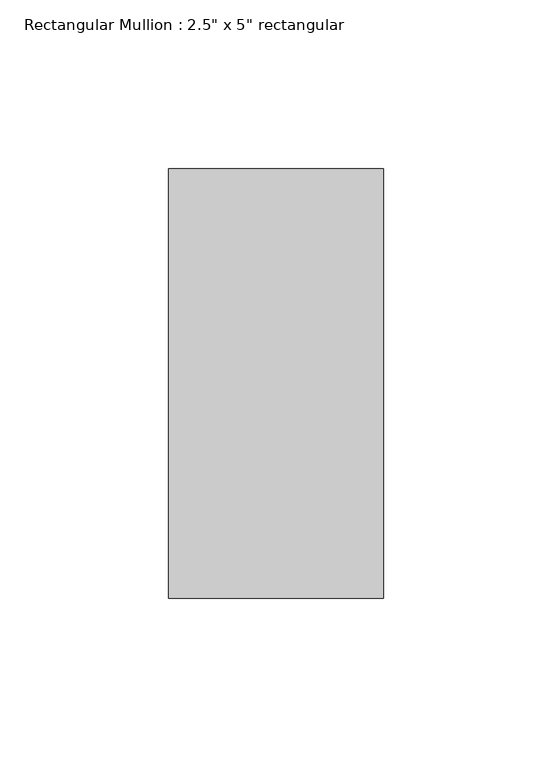
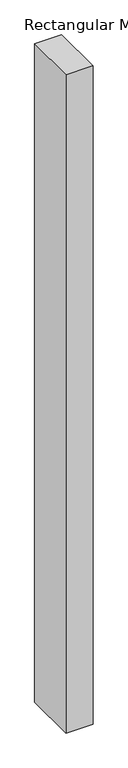
"""IFC4 building model written with IfcOpenShell, lengths in millimetres: member geometry."""

from ifc_helpers import new_model, si_unit, frame, origin, place, context, project, spatial, polyline, outline, extrude, source, transform, mapped, element, save


def member_8f1a2d85(model_context):
    return source(origin(), model_context, "Body", "SweptSolid", [
        extrude(outline(polyline([(0.0, 63.5), (0.0, -63.5), (-63.5, -63.5), (-63.5, 63.5), (0.0, 63.5)])), frame((0.0, 0.0, -1634.2331996), z_axis=(0.0, 0.0, 1.0), x_axis=(1.0, 0.0, 0.0)), (0.0, 0.0, 1.0), 1634.2331996),
    ])


if __name__ == "__main__":
    model = new_model("IFC4")
    model_context = context("Model", 3, world=origin())
    ifc_project = project(units=[si_unit("LENGTHUNIT", "METRE", prefix="MILLI")], contexts=[model_context])
    site = spatial("IfcSite", under=ifc_project)
    building = spatial("IfcBuilding", under=site)
    placement = place(None, origin())
    member_shape = member_8f1a2d85(model_context)
    element("IfcMember", 1, ObjectType="Rectangular Mullion : 2.5\" x 5\" rectangular", at=placement, inside=building, context=model_context, shape_type="MappedRepresentation", body=[
        mapped(member_shape, transform((0.0, 0.0, 0.0), x_axis=(1.0, 0.0, 0.0), y_axis=(0.0, 1.0, 0.0), z_axis=(0.0, 0.0, 1.0))),
    ])
    save(model, "model.ifc")

# Revit data of these elements
# Type "Rectangular Mullion : 2.5\" x 5\" rectangular"
#   built-in parameter 1007304 = 0.416667 (stored number, unit not read)
#   built-in parameter 1007301 = 0.104167 (stored number, unit not read)
#   built-in parameter 1007300 = 0.104167 (stored number, unit not read)
# Element 1 (IfcMember, "Rectangular Mullion : 2.5\" x 5\" rectangular")
#   Materials on its faces: "Aluminum"
# Materials
#   "Aluminum": class "Metal", colour RGB 247 247 247, transparency 0, Description = "Aluminum 6061", Cost = 0
